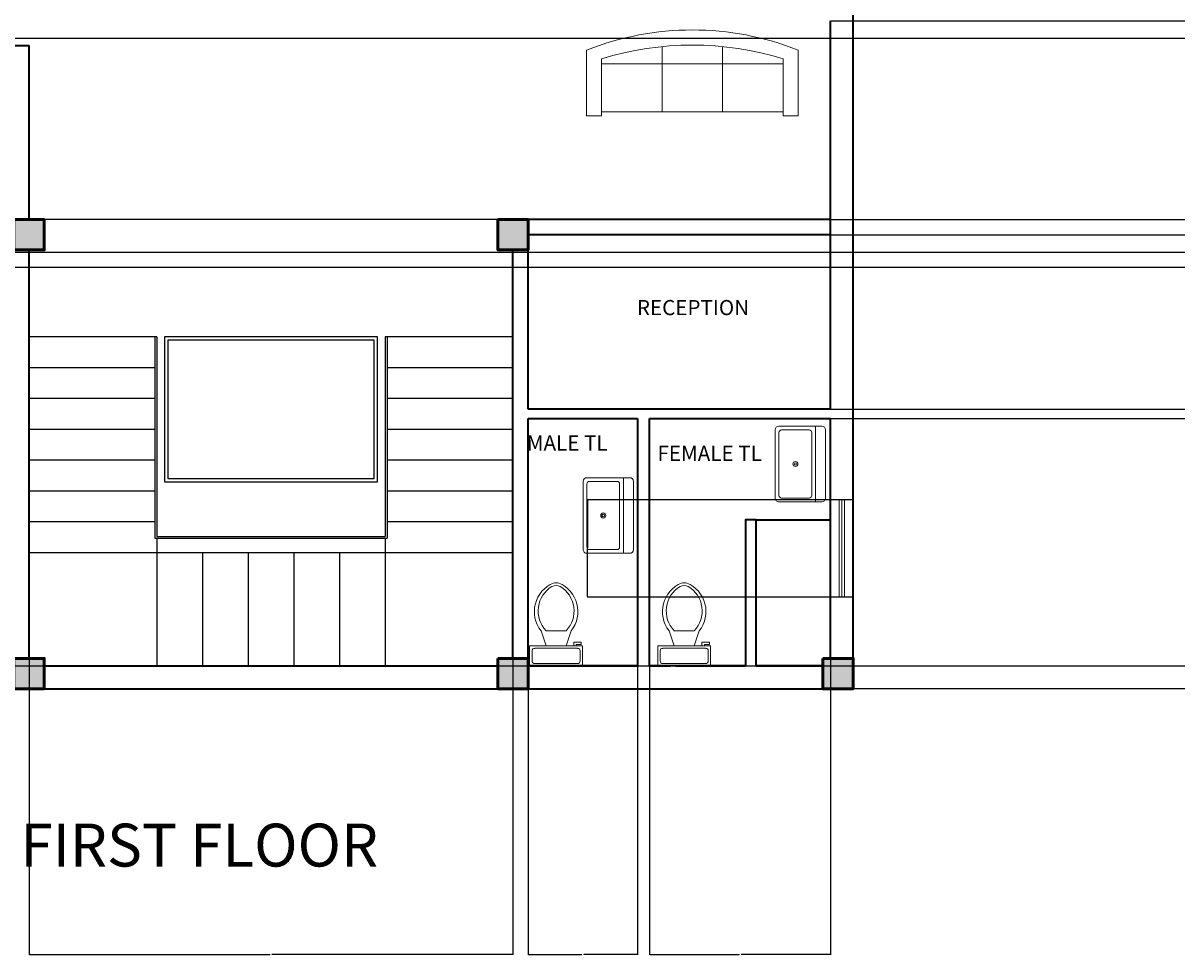
# Model space of a CAD drawing. Units: inches. Extents: x 369 to 4994, y 516 to 1297.
# Tile 5 of 9: x 1452 to 1910, y 516 to 886. Entities that reach past the tile are written whole.
import ezdxf

# ---------------------------------------------------------------- set-up
doc = ezdxf.new("R2010")
doc.units = ezdxf.units.IN
doc.header["$MEASUREMENT"] = 0
for name, color, linetype, lineweight in [('A-ANNO-DIMS', 2, 'Continuous', 18), ('A-ANNO-TEXT', 7, 'Continuous', 35), ('A-AREA-IDEN', 7, 'Continuous', 18), ('A-COLS', 7, 'Continuous', 50), ('A-FLOR-FIXT', 9, 'Continuous', 18), ('A-FLOR-STRS', 3, 'Continuous', 25), ('A-FURN', 8, 'Continuous', 18), ('A-GLAZ', 4, 'Continuous', 18), ('A-WALL', 7, 'Continuous', 35)]:
    doc.layers.add(name, color=color, linetype=linetype, lineweight=lineweight)
doc.layers.add('A-COLS-PATT', color=18, linetype='Continuous', lineweight=13, true_color=0x000000)
doc.styles.get("Standard").update_dxf_attribs({"font": 'arial.ttf'})
doc.dimstyles.get("Standard").update_dxf_attribs({"dimtxt": 0.18, "dimasz": 0.18, "dimexe": 0.18, "dimexo": 0.0625, "dimgap": 0.09, "dimtad": 0, "dimtih": 1, "dimtoh": 1, "dimdec": 4, "dimzin": 0, "dimdsep": 46, "dimtxsty": 'Standard', "dimcen": 0.09, "dimadec": 0, "dimazin": 0, "dimtfac": 1, "dimtdec": 4, "dimtofl": 0, "dimtmove": 0, "dimatfit": 3, "dimfxl": 1, "dimtolj": 1, "dimtzin": 0, "dimarcsym": 0})

# ---------------------------------------------------------------- blocks, each defined once
blk = doc.blocks.new('Sofa - Roundback 7 ft.')
for p, q in [((-12.00002, -32.4421), (-12.00003, -6.5971)), ((11.99997, -32.4421), (11.99998, -6.5971)), ((-36.000027, -34), (-36.000027, -11.4696)), ((-35.999844, -13.3819), (35.9998, -13.3819)), ((35.99998, -34), (35.99998, -11.4696)), ((-36.000027, -32.4421), (35.99998, -32.4421))]:
    blk.add_line(p, q)
for points in [[(-36.000027, -34), (-42.000027, -34), (-42.000027, -8)], [(41.99998, -8), (41.99998, -34), (35.99998, -34)]]:
    blk.add_lwpolyline(points)
for centre, radius, start, end in [((0, -114.25), 114.25, 68.43141, 111.5686), ((-0.00001, -127.1968), 121.1968, 72.72033, 107.2797)]:
    blk.add_arc(centre, radius, start, end)
blk = doc.blocks.new('Sink-single - 30 in top')
blk.add_line((-15, -3.999996), (15, -3.999996))
for points in [[(-13.5, 0), (13.5, 0)], [(-15, -18.499996), (-15, -1.5)], [(15, -1.5), (15, -18.499996)], [(-13.5, -17.499996), (-13.5, -6.499996)], [(-12.5, -5.499996), (12.5, -5.499996)], [(13.5, -6.499996), (13.5, -17.499996)], [(13.5, -19.999996), (-13.5, -19.999996)], [(12.5, -18.499996), (-12.5, -18.499996)]]:
    blk.add_lwpolyline(points)
for radius in [1, 0.5]:
    blk.add_circle((0, -11.999996), radius)
for centre, radius, start, end in [((-13.5, -1.5), 1.5, 90, 180), ((13.5, -1.5), 1.5, 0, 90), ((-12.5, -6.499996), 1, 90, 180), ((12.5, -6.499996), 1, 0, 90), ((-12.5, -17.499996), 1, 180, 270), ((12.5, -17.499996), 1, 270, 0), ((-13.5, -18.499996), 1.5, 180, 270), ((13.5, -18.499996), 1.5, 270, 0)]:
    blk.add_arc(centre, radius, start, end)
blk = doc.blocks.new('Toilet - top')
for p, q in [((9.5, -6), (9.5, -2)), ((-10, -8.5), (-8, -8.5)), ((-10, -9.5), (-10, -8.5)), ((-8, -8.5), (-8, -8)), ((-7, -8), (-7, -9.5)), ((-4, -8), (-6, -14)), ((4, -8), (6, -14)), ((-7, -9.5), (-10, -9.5)), ((4, -14), (-4, -14))]:
    blk.add_line(p, q)
blk.add_lwpolyline([(10.5, -8), (10.5, 0), (-10.5, 0), (-10.5, -8)], close=True)
for points in [[(-9.5, -2), (-9.5, -6)], [(8.5, -1), (-8.5, -1)], [(-8.5, -7), (8.5, -7)]]:
    blk.add_lwpolyline(points)
for centre, radius, start, end in [((-8.62, -1.88), 0.884, 81.8699, 188.1301), ((8.62, -1.88), 0.884, 351.8699, 98.1301), ((-8.62, -6.12), 0.884, 171.8699, 278.1301), ((8.62, -6.12), 0.884, 261.8699, 8.1301), ((3.52, -21.58), 12.17, 141.4691, 247.9714), ((4.2, -21.82), 11.33, 136.3677, 238.9468), ((-3.52, -21.58), 12.17, 292.0284, 38.5307), ((-4.2, -21.82), 11.33, 301.053, 43.6321), ((0, -27.88), 4, 245.7318, 294.2682), ((0, -29), 4, 254.8605, 285.1395)]:
    blk.add_arc(centre, radius, start, end)
blk = doc.blocks.new('STAIR-WELL-FRAME')
for p, q in [((0, 57.51), (0, 0)), ((84.51, 57.51), (0, 57.51)), ((83.15, 56.15), (1.36, 56.15)), ((1.36, 56.15), (1.36, 1.36)), ((83.15, 1.36), (83.15, 56.15)), ((84.51, 0), (84.51, 57.51)), ((84.51, 0), (84.51, 57.51)), ((1.36, 1.36), (83.15, 1.36)), ((0, 0), (84.51, 0))]:
    blk.add_line(p, q)
blk = doc.blocks.new('*D47')
at = {"layer": 'A-ANNO-DIMS', "color": 0, "lineweight": -2, "transparency": 16777216}
for p, q in [((1038.32, 879.79), (2671.51, 879.79)), ((2671.33, 879.61), (2671.33, 837.52)), ((2671.33, 795.07), (2671.33, 837.16)), ((1035.32, 794.89), (2671.51, 794.89))]:
    blk.add_line(p, q, dxfattribs=at)
at = {"layer": 'A-ANNO-DIMS', "color": 0, "transparency": 16777216}
for points in [[(2671.3, 879.61), (2671.36, 879.61), (2671.33, 879.79)], [(2671.3, 795.07), (2671.36, 795.07), (2671.33, 794.89)]]:
    blk.add_solid(points, dxfattribs=at)
at = {"layer": 'Defpoints', "color": 0, "transparency": 16777216}
for p in [(1038.26, 879.79), (2671.33, 879.79), (1035.26, 794.89)]:
    blk.add_point(p, dxfattribs=at)
at = {"layer": 'A-ANNO-DIMS', "color": 0, "transparency": 16777216, "insert": (2671.33, 837.34), "char_height": 0.18, "attachment_point": 5}
blk.add_mtext('\\A1;84.9', dxfattribs=at)
blk = doc.blocks.new('*D52')
at = {"layer": 'A-ANNO-DIMS', "color": 0, "lineweight": -2, "transparency": 16777216}
for p, q in [((942.32, 788.89), (2671.51, 788.89)), ((2671.33, 788.71), (2671.33, 710.02)), ((2671.33, 630.97), (2671.33, 709.66)), ((1035.32, 630.79), (2671.51, 630.79))]:
    blk.add_line(p, q, dxfattribs=at)
at = {"layer": 'A-ANNO-DIMS', "color": 0, "transparency": 16777216}
for points in [[(2671.3, 788.71), (2671.36, 788.71), (2671.33, 788.89)], [(2671.3, 630.97), (2671.36, 630.97), (2671.33, 630.79)]]:
    blk.add_solid(points, dxfattribs=at)
at = {"layer": 'Defpoints', "color": 0, "transparency": 16777216}
for p in [(942.26, 788.89), (2671.33, 788.89), (1035.26, 630.79)]:
    blk.add_point(p, dxfattribs=at)
at = {"layer": 'A-ANNO-DIMS', "color": 0, "transparency": 16777216, "insert": (2671.33, 709.84), "char_height": 0.18, "attachment_point": 5}
blk.add_mtext('\\A1;158.1', dxfattribs=at)
blk = doc.blocks.new('*D80')
at = {"layer": 'A-ANNO-DIMS', "color": 0, "lineweight": -2, "transparency": 16777216}
for p, q in [((1772.44, 886.6), (2671.51, 886.6)), ((2671.33, 886.42), (2671.33, 847.38)), ((2671.33, 807.97), (2671.33, 847.01)), ((1772.44, 807.79), (2671.51, 807.79))]:
    blk.add_line(p, q, dxfattribs=at)
at = {"layer": 'A-ANNO-DIMS', "color": 0, "transparency": 16777216}
for points in [[(2671.3, 886.42), (2671.36, 886.42), (2671.33, 886.6)], [(2671.3, 807.97), (2671.36, 807.97), (2671.33, 807.79)]]:
    blk.add_solid(points, dxfattribs=at)
at = {"layer": 'Defpoints', "color": 0, "transparency": 16777216}
for p in [(1772.37, 886.6), (2671.33, 886.6), (1772.37, 807.79)]:
    blk.add_point(p, dxfattribs=at)
at = {"layer": 'A-ANNO-DIMS', "color": 0, "transparency": 16777216, "insert": (2671.33, 847.19), "char_height": 0.18, "attachment_point": 5}
blk.add_mtext('\\A1;78.81', dxfattribs=at)
blk = doc.blocks.new('*D82')
at = {"layer": 'A-ANNO-DIMS', "color": 0, "lineweight": -2, "transparency": 16777216}
for p, q in [((1454.37, 761.23), (1454.37, 516.21)), ((1646.37, 761.23), (1646.37, 516.21)), ((1454.55, 516.39), (1550.09, 516.39)), ((1646.19, 516.39), (1550.65, 516.39))]:
    blk.add_line(p, q, dxfattribs=at)
at = {"layer": 'A-ANNO-DIMS', "color": 0, "transparency": 16777216}
for points in [[(1454.55, 516.42), (1454.55, 516.36), (1454.37, 516.39)], [(1646.19, 516.42), (1646.19, 516.36), (1646.37, 516.39)]]:
    blk.add_solid(points, dxfattribs=at)
at = {"layer": 'Defpoints', "color": 0, "transparency": 16777216}
for p in [(1454.37, 761.29), (1646.37, 761.29), (1646.37, 516.39)]:
    blk.add_point(p, dxfattribs=at)
at = {"layer": 'A-ANNO-DIMS', "color": 0, "transparency": 16777216, "insert": (1550.37, 516.39), "char_height": 0.18, "attachment_point": 5}
blk.add_mtext('\\A1;192', dxfattribs=at)
blk = doc.blocks.new('*D83')
at = {"layer": 'A-ANNO-DIMS', "color": 0, "lineweight": -2, "transparency": 16777216}
for p, q in [((1652.37, 630.73), (1652.37, 516.21)), ((1695.8, 630.73), (1695.8, 516.21)), ((1652.55, 516.39), (1673.69, 516.39)), ((1695.62, 516.39), (1674.49, 516.39))]:
    blk.add_line(p, q, dxfattribs=at)
at = {"layer": 'A-ANNO-DIMS', "color": 0, "transparency": 16777216}
for points in [[(1652.55, 516.42), (1652.55, 516.36), (1652.37, 516.39)], [(1695.62, 516.42), (1695.62, 516.36), (1695.8, 516.39)]]:
    blk.add_solid(points, dxfattribs=at)
at = {"layer": 'Defpoints', "color": 0, "transparency": 16777216}
for p in [(1652.37, 630.79), (1695.8, 630.79), (1695.8, 516.39)]:
    blk.add_point(p, dxfattribs=at)
at = {"layer": 'A-ANNO-DIMS', "color": 0, "transparency": 16777216, "insert": (1674.09, 516.39), "char_height": 0.18, "attachment_point": 5}
blk.add_mtext('\\A1;43.43', dxfattribs=at)
blk = doc.blocks.new('*D84')
at = {"layer": 'A-ANNO-DIMS', "color": 0, "lineweight": -2, "transparency": 16777216}
for p, q in [((1700.59, 728.91), (1700.59, 516.21)), ((1772.37, 728.91), (1772.37, 516.21)), ((1700.77, 516.39), (1736.09, 516.39)), ((1772.19, 516.39), (1736.87, 516.39))]:
    blk.add_line(p, q, dxfattribs=at)
at = {"layer": 'A-ANNO-DIMS', "color": 0, "transparency": 16777216}
for points in [[(1700.77, 516.42), (1700.77, 516.36), (1700.59, 516.39)], [(1772.19, 516.42), (1772.19, 516.36), (1772.37, 516.39)]]:
    blk.add_solid(points, dxfattribs=at)
at = {"layer": 'Defpoints', "color": 0, "transparency": 16777216}
for p in [(1700.59, 728.97), (1772.37, 728.97), (1772.37, 516.39)]:
    blk.add_point(p, dxfattribs=at)
at = {"layer": 'A-ANNO-DIMS', "color": 0, "transparency": 16777216, "insert": (1736.48, 516.39), "char_height": 0.18, "attachment_point": 5}
blk.add_mtext('\\A1;71.79', dxfattribs=at)
blk = doc.blocks.new('*D85')
at = {"layer": 'A-ANNO-DIMS', "color": 0, "lineweight": -2, "transparency": 16777216}
for p, q in [((1772.44, 801.79), (2671.51, 801.79)), ((2671.33, 801.61), (2671.33, 767.36)), ((2671.33, 732.75), (2671.33, 767)), ((1772.44, 732.57), (2671.51, 732.57))]:
    blk.add_line(p, q, dxfattribs=at)
at = {"layer": 'A-ANNO-DIMS', "color": 0, "transparency": 16777216}
for points in [[(2671.3, 801.61), (2671.36, 801.61), (2671.33, 801.79)], [(2671.3, 732.75), (2671.36, 732.75), (2671.33, 732.57)]]:
    blk.add_solid(points, dxfattribs=at)
at = {"layer": 'Defpoints', "color": 0, "transparency": 16777216}
for p in [(1772.37, 801.79), (2671.33, 801.79), (1772.37, 732.57)]:
    blk.add_point(p, dxfattribs=at)
at = {"layer": 'A-ANNO-DIMS', "color": 0, "transparency": 16777216, "insert": (2671.33, 767.18), "char_height": 0.18, "attachment_point": 5}
blk.add_mtext('\\A1;69.22', dxfattribs=at)
blk = doc.blocks.new('*D86')
at = {"layer": 'A-ANNO-DIMS', "color": 0, "lineweight": -2, "transparency": 16777216}
for p, q in [((1772.44, 728.97), (2671.51, 728.97)), ((2671.33, 728.79), (2671.33, 680.06)), ((2671.33, 630.97), (2671.33, 679.7)), ((1769.44, 630.79), (2671.51, 630.79))]:
    blk.add_line(p, q, dxfattribs=at)
at = {"layer": 'A-ANNO-DIMS', "color": 0, "transparency": 16777216}
for points in [[(2671.3, 728.79), (2671.36, 728.79), (2671.33, 728.97)], [(2671.3, 630.97), (2671.36, 630.97), (2671.33, 630.79)]]:
    blk.add_solid(points, dxfattribs=at)
at = {"layer": 'Defpoints', "color": 0, "transparency": 16777216}
for p in [(1772.37, 728.97), (2671.33, 728.97), (1769.37, 630.79)]:
    blk.add_point(p, dxfattribs=at)
at = {"layer": 'A-ANNO-DIMS', "color": 0, "transparency": 16777216, "insert": (2671.33, 679.88), "char_height": 0.18, "attachment_point": 5}
blk.add_mtext('\\A1;98.18', dxfattribs=at)
blk = doc.blocks.new('*D88')
at = {"layer": 'A-ANNO-DIMS', "color": 0, "lineweight": -2, "transparency": 16777216}
for p, q in [((1390.27, 870.84), (1446.63, 960.04)), ((1446.68, 959.8), (1460.49, 951.07)), ((1474.87, 941.99), (1461.06, 950.71)), ((1418.75, 852.84), (1475.12, 942.04))]:
    blk.add_line(p, q, dxfattribs=at)
at = {"layer": 'A-ANNO-DIMS', "color": 0, "transparency": 16777216}
for points in [[(1446.7, 959.82), (1446.67, 959.77), (1446.53, 959.89)], [(1474.88, 942.01), (1474.85, 941.96), (1475.02, 941.89)]]:
    blk.add_solid(points, dxfattribs=at)
at = {"layer": 'Defpoints', "color": 0, "transparency": 16777216}
for p in [(1475.02, 941.89), (1390.23, 870.79), (1418.72, 852.79)]:
    blk.add_point(p, dxfattribs=at)
at = {"layer": 'A-ANNO-DIMS', "color": 0, "transparency": 16777216, "insert": (1460.78, 950.89), "char_height": 0.18, "attachment_point": 5}
blk.add_mtext('\\A1;33.7', dxfattribs=at)
blk = doc.blocks.new('*D96')
at = {"layer": 'A-ANNO-DIMS', "color": 0, "lineweight": -2, "transparency": 16777216}
for p, q in [((1781.31, 696.73), (1675.79, 696.73)), ((1675.97, 696.55), (1675.97, 677.61)), ((1675.97, 658.31), (1675.97, 677.25)), ((1781.31, 658.13), (1675.79, 658.13))]:
    blk.add_line(p, q, dxfattribs=at)
at = {"layer": 'A-ANNO-DIMS', "color": 0, "transparency": 16777216}
for points in [[(1675.94, 696.55), (1676, 696.55), (1675.97, 696.73)], [(1675.94, 658.31), (1676, 658.31), (1675.97, 658.13)]]:
    blk.add_solid(points, dxfattribs=at)
at = {"layer": 'Defpoints', "color": 0, "transparency": 16777216}
for p in [(1675.97, 696.73), (1781.37, 696.73), (1781.37, 658.13)]:
    blk.add_point(p, dxfattribs=at)
at = {"layer": 'A-ANNO-DIMS', "color": 0, "transparency": 16777216, "insert": (1675.97, 677.43), "char_height": 0.18, "attachment_point": 5}
blk.add_mtext('\\A1;38.6', dxfattribs=at)
blk = doc.blocks.new('*D98')
at = {"layer": 'A-ANNO-DIMS', "color": 0, "lineweight": -2, "transparency": 16777216}
for p, q in [((1992.86, 1038.79), (368.68, 1038.79)), ((368.86, 1038.61), (368.86, 830.47)), ((368.86, 621.97), (368.86, 830.11)), ((2046.86, 621.79), (368.68, 621.79))]:
    blk.add_line(p, q, dxfattribs=at)
at = {"layer": 'A-ANNO-DIMS', "color": 0, "transparency": 16777216}
for points in [[(368.83, 1038.61), (368.89, 1038.61), (368.86, 1038.79)], [(368.83, 621.97), (368.89, 621.97), (368.86, 621.79)]]:
    blk.add_solid(points, dxfattribs=at)
at = {"layer": 'Defpoints', "color": 0, "transparency": 16777216}
for p in [(368.86, 1038.79), (1992.93, 1038.79), (2046.93, 621.79)]:
    blk.add_point(p, dxfattribs=at)
at = {"layer": 'A-ANNO-DIMS', "color": 0, "transparency": 16777216, "insert": (368.86, 830.29), "char_height": 0.18, "attachment_point": 5}
blk.add_mtext('\\A1;417', dxfattribs=at)

msp = doc.modelspace()

# ---------------------------------------------------------------- hatches: boundary and pattern name
at = {"layer": 'A-COLS-PATT'}
h = msp.add_hatch(color=256, dxfattribs=at)
h.dxf.hatch_style = 1
h.paths.add_polyline_path([(540.2581, 633.7894), (528.2581, 633.7894), (528.2581, 621.7894), (540.2581, 621.7894)])
h.paths.add_polyline_path([(726.2581, 633.7894), (714.2581, 633.7894), (714.2581, 621.7894), (726.2581, 621.7894)])
h.paths.add_polyline_path([(918.2581, 633.7894), (906.2581, 633.7894), (906.2581, 621.7894), (918.2581, 621.7894)])
h.paths.add_polyline_path([(1047.2581, 633.7894), (1035.2581, 633.7894), (1035.2581, 621.7894), (1047.2581, 621.7894)])
h.paths.add_polyline_path([(1047.2581, 798.6977), (1035.2581, 798.6977), (1035.2581, 786.6977), (1047.2581, 786.6977)])
h.paths.add_polyline_path([(918.2581, 795.7894), (906.2581, 795.7894), (906.2581, 783.7894), (918.2581, 783.7894)])
h.paths.add_polyline_path([(726.2581, 795.7894), (714.2581, 795.7894), (714.2581, 783.7894), (726.2581, 783.7894)])
h.paths.add_polyline_path([(1047.2581, 1038.7894), (1035.2581, 1038.7894), (1035.2581, 1026.7894), (1047.2581, 1026.7894)])
h.paths.add_polyline_path([(855.044, 1038.7894), (843.044, 1038.7894), (843.044, 1026.7894), (855.044, 1026.7894)])
h.paths.add_polyline_path([(728.5536, 1038.7894), (716.5536, 1038.7894), (716.5536, 1026.7894), (728.5536, 1026.7894)])
h.paths.add_polyline_path([(543.2581, 1038.7894), (531.2581, 1038.7894), (531.2581, 1026.7894), (543.2581, 1026.7894)])
h.paths.add_polyline_path([(543.2581, 792.9013), (531.2581, 792.9013), (531.2581, 780.9013), (543.2581, 780.9013), (543.2581, 783.7894)])
h.paths.add_polyline_path([(1274.3738, 633.7894), (1262.3738, 633.7894), (1262.3738, 621.7894), (1274.3738, 621.7894)])
h.paths.add_polyline_path([(1460.3738, 633.7894), (1448.3738, 633.7894), (1448.3738, 621.7894), (1460.3738, 621.7894)])
h.paths.add_polyline_path([(1652.3738, 633.7894), (1640.3738, 633.7894), (1640.3738, 621.7894), (1652.3738, 621.7894)])
h.paths.add_polyline_path([(1781.3738, 633.7894), (1769.3738, 633.7894), (1769.3738, 621.7894), (1781.3738, 621.7894)])
h.paths.add_polyline_path([(1781.3738, 1038.7894), (1769.3738, 1038.7894), (1769.3738, 1026.7894), (1781.3738, 1026.7894)])
h.paths.add_polyline_path([(1625.484, 1038.7894), (1613.484, 1038.7894), (1613.484, 1026.7894), (1615.6962, 1026.7894), (1625.484, 1026.7894)])
h.paths.add_polyline_path([(1462.6692, 1038.7894), (1450.6692, 1038.7894), (1450.6692, 1026.7894), (1462.6692, 1026.7894)])
h.paths.add_polyline_path([(1277.3738, 1038.7894), (1265.3738, 1038.7894), (1265.3738, 1026.7894), (1277.3738, 1026.7894)])
h.paths.add_polyline_path([(1460.3738, 807.7894), (1448.3738, 807.7894), (1448.3738, 795.7894), (1460.3738, 795.7894)])
h.paths.add_polyline_path([(1652.3738, 807.7894), (1640.3738, 807.7894), (1640.3738, 795.7894), (1652.3738, 795.7894)])
h.paths.add_polyline_path([(2244.9265, 633.7894), (2232.9265, 633.7894), (2232.9265, 621.7894), (2244.9265, 621.7894)])
h.paths.add_polyline_path([(2058.9265, 633.7894), (2046.9265, 633.7894), (2046.9265, 621.7894), (2058.9265, 621.7894)])
h.paths.add_polyline_path([(2436.9265, 633.7894), (2424.9265, 633.7894), (2424.9265, 621.7894), (2436.9265, 621.7894)])
h.paths.add_polyline_path([(2565.9265, 633.7894), (2553.9265, 633.7894), (2553.9265, 621.7894), (2565.9265, 621.7894)])
h.paths.add_polyline_path([(2565.9265, 798.6977), (2553.9265, 798.6977), (2553.9265, 786.6977), (2565.9265, 786.6977)])
h.paths.add_polyline_path([(2565.9265, 1038.7894), (2553.9265, 1038.7894), (2553.9265, 1026.7894), (2565.9265, 1026.7894)])
h.paths.add_polyline_path([(2436.9265, 1038.7894), (2424.9265, 1038.7894), (2424.9265, 1026.7894), (2436.9265, 1026.7894)])
h.paths.add_polyline_path([(2247.222, 1038.7894), (2235.222, 1038.7894), (2235.222, 1026.7894), (2247.222, 1026.7894)])
h.paths.add_polyline_path([(2061.9265, 1038.7894), (2049.9265, 1038.7894), (2049.9265, 1026.7894), (2061.9265, 1026.7894)])

# ---------------------------------------------------------------- linework, layer by layer
at = {"layer": 'A-COLS'}
for points in [[(1448.3738, 807.7894), (1460.3738, 807.7894), (1460.3738, 795.7894), (1448.3738, 795.7894)], [(1640.3738, 807.7894), (1652.3738, 807.7894), (1652.3738, 795.7894), (1640.3738, 795.7894)], [(1448.3738, 633.7894), (1460.3738, 633.7894), (1460.3738, 621.7894), (1448.3738, 621.7894)], [(1640.3738, 633.7894), (1652.3738, 633.7894), (1652.3738, 621.7894), (1640.3738, 621.7894)], [(1769.3738, 633.7894), (1781.3738, 633.7894), (1781.3738, 621.7894), (1769.3738, 621.7894)]]:
    msp.add_lwpolyline(points, close=True, dxfattribs=at)
at = {"layer": 'A-FLOR-STRS'}
for p, q in [((1640.3738, 807.7894), (1460.3738, 807.7894)), ((1505.0379, 761.2935), (1454.3738, 761.2935)), ((1504.322, 761.2935), (1504.322, 681.4595)), ((1505.0379, 761.2935), (1505.0379, 682.1754)), ((1646.3738, 761.2935), (1595.7097, 761.2935)), ((1595.7097, 761.2935), (1595.7097, 682.1754)), ((1596.4256, 761.2935), (1596.4256, 681.4595)), ((1504.322, 749.0604), (1454.3738, 749.0604)), ((1646.3738, 749.0604), (1596.4256, 749.0604)), ((1504.322, 736.8273), (1454.3738, 736.8273)), ((1646.3738, 736.8273), (1596.4256, 736.8273)), ((1504.322, 724.5942), (1454.3738, 724.5942)), ((1646.3738, 724.5942), (1596.4256, 724.5942)), ((1504.322, 712.361), (1454.3738, 712.361)), ((1646.3738, 712.361), (1596.4256, 712.361)), ((1504.322, 700.1279), (1454.3738, 700.1279)), ((1646.3738, 700.1279), (1596.4256, 700.1279)), ((1504.322, 687.8948), (1454.3738, 687.8948)), ((1646.3738, 687.8948), (1596.4256, 687.8948)), ((1505.0379, 682.1754), (1595.7097, 682.1754)), ((1504.322, 681.4595), (1596.4256, 681.4595)), ((1505.0379, 681.4595), (1505.0379, 630.7894)), ((1595.7097, 681.4595), (1595.7097, 630.7894)), ((1646.3738, 675.6617), (1454.3738, 675.6617)), ((1523.1723, 675.6617), (1523.1723, 630.7894)), ((1541.3066, 675.6617), (1541.3066, 630.7894)), ((1559.441, 675.6617), (1559.441, 630.7894)), ((1577.5754, 675.6617), (1577.5754, 630.7894)), ((1595.7097, 675.6617), (1595.7097, 630.7894))]:
    msp.add_line(p, q, dxfattribs=at)
at = {"layer": 'A-GLAZ'}
for p, q in [((1775.7977, 696.7316), (1775.7977, 658.1309)), ((1776.8738, 696.7316), (1776.8738, 658.1309)), ((1777.9499, 696.7316), (1777.9499, 658.1309))]:
    msp.add_line(p, q, dxfattribs=at)
msp.add_lwpolyline([(1772.3738, 658.1309), (1781.3738, 658.1309), (1781.3738, 696.7316), (1772.3738, 696.7316)], close=True, dxfattribs=at)
at = {"layer": 'A-WALL'}
for p, q in [((1781.3738, 621.7894), (1781.3738, 1029.7894)), ((1772.3738, 732.5675), (1772.3738, 886.5988)), ((1448.3738, 876.7894), (1454.3738, 876.7894)), ((1454.3738, 870.7894), (1454.3738, 876.7894)), ((1454.3738, 807.7894), (1454.3738, 870.7894)), ((1772.3738, 807.7894), (1652.3738, 807.7894)), ((1772.3738, 801.7894), (1652.3738, 801.7894)), ((1454.3738, 633.7894), (1454.3738, 795.7894)), ((1646.3738, 633.7894), (1646.3738, 795.7894)), ((1652.3738, 792.6977), (1652.3738, 795.7894)), ((1652.3738, 732.5675), (1652.3738, 795.7894)), ((1772.3738, 771.7894), (1772.3738, 786.6977)), ((1772.3738, 732.5675), (1772.3738, 786.6977)), ((1772.3738, 732.5675), (1772.3738, 786.6977)), ((1652.3738, 633.7894), (1652.3738, 728.9712)), ((1772.3738, 633.7894), (1772.3738, 728.9712)), ((1772.3738, 633.7894), (1772.3738, 728.9712)), ((1742.8859, 688.7507), (1772.3738, 688.7507)), ((1460.3738, 630.7894), (1640.3738, 630.7894)), ((1652.3738, 630.7894), (1695.8026, 630.7894)), ((1695.8026, 630.7894), (1652.3738, 630.7894)), ((1695.8026, 630.7894), (1652.3738, 630.7894)), ((1708.8738, 630.7894), (1700.5885, 630.7894)), ((1738.6446, 630.7894), (1700.5885, 630.7894)), ((1700.5885, 630.7894), (1708.8738, 630.7894)), ((1738.6446, 630.7894), (1710.8738, 630.7894)), ((1710.8738, 630.7894), (1738.6446, 630.7894)), ((1769.3738, 630.7894), (1742.8859, 630.7894)), ((1742.8859, 630.7894), (1769.3738, 630.7894)), ((1460.3738, 621.7894), (1652.3738, 621.7894)), ((1652.3738, 621.7894), (1781.3738, 621.7894))]:
    msp.add_line(p, q, dxfattribs=at)
for points in [[(1772.3738, 732.5675), (1652.3738, 732.5675)], [(1652.3738, 728.9712), (1695.8026, 728.9712)], [(1695.8026, 728.9712), (1695.8026, 630.7894)], [(1700.5885, 630.7894), (1700.5885, 728.9712)], [(1700.5885, 728.9712), (1772.3738, 728.9712)], [(1742.8859, 630.7894), (1742.8859, 688.7507), (1738.6446, 688.7507), (1738.6446, 630.7894)]]:
    msp.add_lwpolyline(points, dxfattribs=at)

# ---------------------------------------------------------------- block references
at = {"layer": 'A-FLOR-FIXT'}
for name, p, rotation in [('Sink-single - 30 in top', (1770.4211, 710.8875), 269.9999999999999), ('Sink-single - 30 in top', (1694.1907, 690.4616), 269.9999999999999), ('Toilet - top', (1663.4917, 630.7894), 180), ('Toilet - top', (1714.3037, 630.7894), 180)]:
    msp.add_blockref(name, p, dxfattribs=dict(at, rotation=rotation))
at = {"layer": 'A-FLOR-STRS'}
msp.add_blockref('STAIR-WELL-FRAME', (1508.1177, 703.781), dxfattribs=at)
at = {"layer": 'A-FURN'}
msp.add_blockref('Sofa - Roundback 7 ft.', (1717.5581, 883.0145), dxfattribs=at)

# ---------------------------------------------------------------- texts
at = {"layer": 'A-ANNO-TEXT'}
msp.add_text('FIRST FLOOR ', height=17.017766, dxfattribs=at).set_placement((1450.9504, 551.2491))
at = {"layer": 'A-AREA-IDEN'}
for s, p in [('RECEPTION', (1695.5285, 769.9223)), ('MALE TL ', (1651.8442, 716.2128)), ('FEMALE TL   ', (1703.6928, 712.1111))]:
    msp.add_text(s, height=6, dxfattribs=at).set_placement(p)

# ---------------------------------------------------------------- dimensions: what is measured, and where the dimension line sits
at = {"layer": 'A-ANNO-DIMS'}
for base, p1, p2, angle, override, picture, middle in [((368.8581, 1038.7894), (2046.9265, 621.7894), (1992.9265, 1038.7894), 90, {"dimdec": 0, "dimlfac": 1, "dimrnd": 0, "dimzin": 0, "dimdsep": 46, "dimlunit": 2}, '*D98', (368.8581, 830.2894)), ((1475.0201, 941.8927), (1390.232, 870.7894), (1418.7195, 852.7894), 327.712989, {"dimdec": 1, "dimlfac": 1, "dimrnd": 0, "dimzin": 0, "dimdsep": 46, "dimlunit": 2}, '*D88', (1460.7763, 950.8927)), ((2671.3265, 886.5988), (1772.3738, 807.7894), (1772.3738, 886.5988), 90, {"dimdec": 2, "dimlfac": 1, "dimrnd": 0, "dimzin": 0, "dimdsep": 46, "dimlunit": 2}, '*D80', (2671.3265, 847.1941)), ((2671.3265, 879.7894), (1035.2581, 794.8925), (1038.2581, 879.7894), 90, {"dimdec": 1, "dimlfac": 1, "dimrnd": 0, "dimzin": 0, "dimdsep": 46, "dimlunit": 2}, '*D47', (2671.3265, 837.3409)), ((2671.3265, 801.7894), (1772.3738, 732.5675), (1772.3738, 801.7894), 90, {"dimdec": 2, "dimlfac": 1, "dimrnd": 0, "dimzin": 0, "dimdsep": 46, "dimlunit": 2}, '*D85', (2671.3265, 767.1784)), ((2671.3265, 788.8925), (1035.2581, 630.7894), (942.2581, 788.8925), 90, {"dimdec": 1, "dimlfac": 1, "dimrnd": 0, "dimzin": 0, "dimdsep": 46, "dimlunit": 2}, '*D52', (2671.3265, 709.8409)), ((2671.3265, 728.9712), (1769.3738, 630.7894), (1772.3738, 728.9712), 90, {"dimdec": 2, "dimlfac": 1, "dimrnd": 0, "dimzin": 0, "dimdsep": 46, "dimlunit": 2}, '*D86', (2671.3265, 679.8803)), ((1675.9738, 696.7316), (1781.3738, 658.1309), (1781.3738, 696.7316), 90, {"dimdec": 1, "dimlfac": 1, "dimrnd": 0, "dimzin": 0, "dimdsep": 46, "dimlunit": 2}, '*D96', (1675.9738, 677.4312))]:
    dim = msp.add_linear_dim(base=base, p1=p1, p2=p2, angle=angle, dimstyle='Standard', override=override, dxfattribs=at)
    dim.commit()
    dim.dimension.update_dxf_attribs({"geometry": picture, "text_midpoint": middle})
for base, p1, p2, override, picture, middle in [((1646.3738, 516.3894), (1454.3738, 761.2935), (1646.3738, 761.2935), {"dimdec": 0, "dimlfac": 1, "dimrnd": 0, "dimzin": 0, "dimdsep": 46, "dimlunit": 2}, '*D82', (1550.3738, 516.3894)), ((1772.3738, 516.3894), (1700.5885, 728.9712), (1772.3738, 728.9712), {"dimdec": 2, "dimlfac": 1, "dimrnd": 0, "dimzin": 0, "dimdsep": 46, "dimlunit": 2}, '*D84', (1736.4812, 516.3894)), ((1695.8026, 516.3894), (1652.3738, 630.7894), (1695.8026, 630.7894), {"dimdec": 2, "dimlfac": 1, "dimrnd": 0, "dimzin": 0, "dimdsep": 46, "dimlunit": 2}, '*D83', (1674.0882, 516.3894))]:
    dim = msp.add_linear_dim(base=base, p1=p1, p2=p2, dimstyle='Standard', override=override, dxfattribs=at)
    dim.commit()
    dim.dimension.update_dxf_attribs({"geometry": picture, "text_midpoint": middle})

doc.saveas('drawing.dxf')
